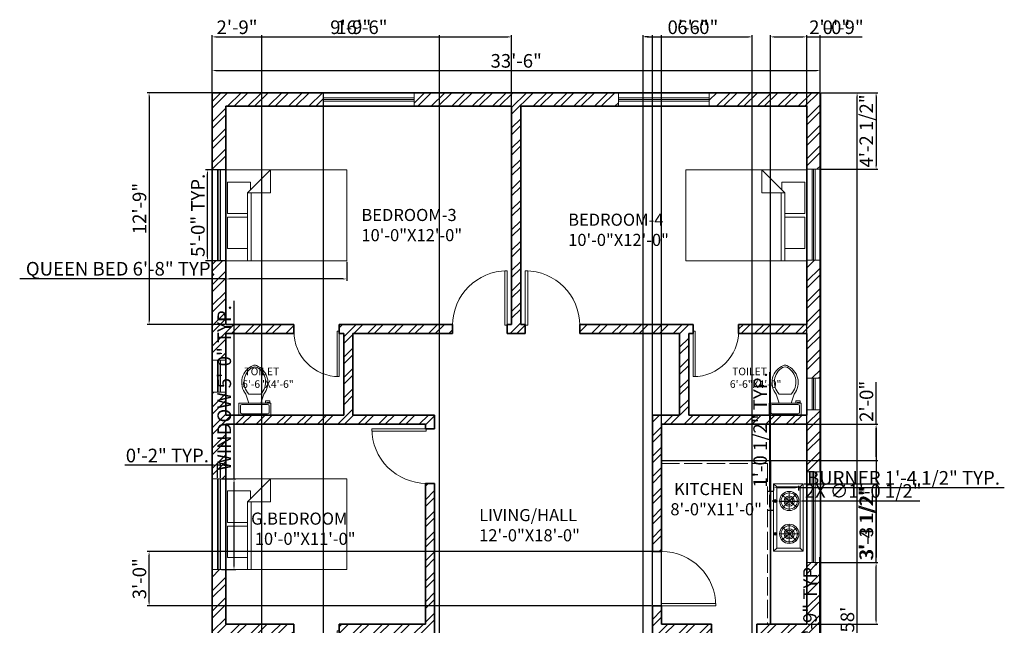
# Model space of a CAD drawing. Units: inches. Extents: x 73 to 724, y 1566 to 2355.
# Tile 2 of 2: x 73 to 724, y 1955 to 2355. Entities that reach past the tile are written whole.
import ezdxf

# ---------------------------------------------------------------- set-up
doc = ezdxf.new("R2010")
doc.units = ezdxf.units.IN
doc.linetypes.add('ACAD_ISO02W100', pattern=[15, 12, -3])
for name, color, linetype, lineweight in [('A-ANNO-DIMS', 2, 'Continuous', 18), ('A-AREA-IDEN', 7, 'Continuous', 18), ('A-DOOR', 4, 'Continuous', 18), ('A-EQPM', 8, 'Continuous', 18), ('A-FLOR-CASE', 9, 'Continuous', 25), ('A-FLOR-CASE-HIDN', 9, 'ACAD_ISO02W100', 13), ('A-FLOR-FIXT', 9, 'Continuous', 18), ('A-FURN', 9, 'Continuous', 18), ('A-GLAZ', 244, 'Continuous', 18), ('A-WALL', 7, 'Continuous', 35), ('A-WALL-PATT', 252, 'Continuous', 13)]:
    doc.layers.add(name, color=color, linetype=linetype, lineweight=lineweight)
doc.styles.get("Standard").update_dxf_attribs({"font": 'arial.ttf'})
doc.dimstyles.new('ISO-25', dxfattribs={"dimtxt": 9, "dimasz": 2.5, "dimexe": 1.25, "dimexo": 0.625, "dimtad": 1, "dimlunit": 3, "dimtxsty": 'Standard', "dimcen": 2.5, "dimadec": 0, "dimazin": 0, "dimtfac": 1, "dimtmove": 0, "dimatfit": 3, "dimfxl": 1, "dimarcsym": 0})

# ---------------------------------------------------------------- blocks, each defined once
blk = doc.blocks.new('*U3')
for p, q in [((0, 0), (0, -6)), ((-40, 0), (-40, -6))]:
    blk.add_line(p, q)
blk.add_lwpolyline([(0, 0), (0, 40), (-1.75, 40), (-1.75, 0)], close=True)
blk.add_arc((0, 0), 40, 90, 180)
blk = doc.blocks.new('*U4')
for p, q in [((0, 0), (0, -6)), ((40, 0), (40, -6))]:
    blk.add_line(p, q)
blk.add_lwpolyline([(0, 0), (0, 40), (1.75, 40), (1.75, 0)], close=True)
blk.add_arc((0, 0), 40, 0, 90)
blk = doc.blocks.new('*U5')
for p, q in [((0, 0), (0, 6)), ((40, 0), (40, 6))]:
    blk.add_line(p, q)
blk.add_lwpolyline([(0, 0), (0, -40), (1.75, -40), (1.75, 0)], close=True)
blk.add_arc((0, 0), 40, 270, 360)
blk = doc.blocks.new('*U6')
for p, q in [((0, 0), (0, 6)), ((40, 0), (40, 6))]:
    blk.add_line(p, q)
blk.add_lwpolyline([(0, 0), (0, -40), (1.75, -40), (1.75, 0)], close=True)
blk.add_arc((0, 0), 40, 270, 0)
blk = doc.blocks.new('*U8')
for p, q in [((-40, 0), (-40, 6)), ((0, 0), (0, 6))]:
    blk.add_line(p, q)
blk.add_lwpolyline([(0, 0), (0, -40), (-1.75, -40), (-1.75, 0)], close=True)
blk.add_arc((0, 0), 40, 180, 270)
blk = doc.blocks.new('*D9')
at = {"layer": 'A-ANNO-DIMS', "color": 0, "lineweight": -2, "transparency": 16777216}
for p, q in [((200.03, 2307.75), (200.03, 2323)), ((202.53, 2321.75), (599.53, 2321.75)), ((602.03, 2307.75), (602.03, 2323))]:
    blk.add_line(p, q, dxfattribs=at)
at = {"layer": 'A-ANNO-DIMS', "color": 0, "transparency": 16777216}
for points in [[(202.53, 2322.17), (202.53, 2321.34), (200.03, 2321.75)], [(599.53, 2322.17), (599.53, 2321.34), (602.03, 2321.75)]]:
    blk.add_solid(points, dxfattribs=at)
at = {"layer": 'Defpoints', "color": 0, "transparency": 16777216}
for p in [(602.03, 2321.75), (200.03, 2307.12), (602.03, 2307.12)]:
    blk.add_point(p, dxfattribs=at)
at = {"layer": 'A-ANNO-DIMS', "color": 0, "transparency": 16777216, "insert": (401.03, 2326.98), "char_height": 9, "attachment_point": 5}
blk.add_mtext('33\'-6"', dxfattribs=at)
blk = doc.blocks.new('*D10')
at = {"layer": 'A-ANNO-DIMS', "color": 0, "lineweight": -2, "transparency": 16777216}
for p, q in [((602.66, 2307.12), (627.57, 2307.12)), ((626.32, 1613.62), (626.32, 2304.62)), ((602.66, 1611.12), (627.57, 1611.12))]:
    blk.add_line(p, q, dxfattribs=at)
at = {"layer": 'A-ANNO-DIMS', "color": 0, "transparency": 16777216}
for points in [[(625.9, 2304.62), (626.74, 2304.62), (626.32, 2307.12)], [(625.9, 1613.62), (626.74, 1613.62), (626.32, 1611.12)]]:
    blk.add_solid(points, dxfattribs=at)
at = {"layer": 'Defpoints', "color": 0, "transparency": 16777216}
for p in [(602.03, 2307.12), (626.32, 2307.12), (602.03, 1611.12)]:
    blk.add_point(p, dxfattribs=at)
at = {"layer": 'A-ANNO-DIMS', "color": 0, "transparency": 16777216, "insert": (621.1, 1959.12), "char_height": 9, "attachment_point": 5, "rotation": 90}
blk.add_mtext("58'", dxfattribs=at)
blk = doc.blocks.new('Bed - Queen')
for p, q in [((0, -80.00003), (0, 0)), ((0, 0), (59.99999, 0)), ((59.99999, 0), (59.99999, -80.00003)), ((7.99999, -1.2), (28.79998, -1.2)), ((7.99999, -14.4), (7.99999, -1.2)), ((28.79998, -1.2), (28.79998, -14.4)), ((31.19999, -1.2), (51.99999, -1.2)), ((31.19999, -14.4), (31.19999, -1.2)), ((51.99999, -1.2), (51.99999, -16.4)), ((0, -14.4), (44.8, -14.4)), ((44.8, -16.8), (0, -16.8)), ((59.99999, -29.6), (44.8, -14.4)), ((44.8, -14.4), (44.8, -29.6)), ((51.99999, -16.4), (46.79936, -16.4)), ((44.8, -29.6), (59.99999, -29.6)), ((59.99999, -80.00003), (0, -80.00003))]:
    blk.add_line(p, q)
blk = doc.blocks.new('*U13')
for p, q in [((9.5, -6), (9.5, -2)), ((-10, -8.5), (-8, -8.5)), ((-10, -9.5), (-10, -8.5)), ((-7, -9.5), (-10, -9.5)), ((-8, -8.5), (-8, -8)), ((-7, -8), (-7, -9.5)), ((-4, -8), (-6, -14)), ((4, -8), (6, -14)), ((4, -14), (-4, -14))]:
    blk.add_line(p, q)
blk.add_lwpolyline([(10.5, -8), (10.5, 0), (-10.5, 0), (-10.5, -8)], close=True)
for points in [[(-9.5, -2), (-9.5, -6)], [(8.5, -1), (-8.5, -1)], [(-8.5, -7), (8.5, -7)]]:
    blk.add_lwpolyline(points)
for centre, radius, start, end in [((-8.62, -1.88), 0.884, 81.8699, 188.1301), ((-8.62, -6.12), 0.884, 171.8699, 278.1301), ((8.62, -1.88), 0.884, 351.8699, 98.1301), ((8.62, -6.12), 0.884, 261.8699, 8.1301), ((3.52, -21.58), 12.17, 141.46911, 247.97143), ((4.2, -21.82), 11.33, 136.36773, 238.94682), ((-3.52, -21.58), 12.17, 292.02843, 38.53071), ((-4.2, -21.82), 11.33, 301.05301, 43.63209), ((0, -27.88), 4, 245.73182, 294.26817), ((0, -29), 4, 254.86053, 285.13947)]:
    blk.add_arc(centre, radius, start, end)
blk = doc.blocks.new('WIN-GLAZING-60IN')
for p, q in [((0, 2), (60, 2)), ((0, 1), (60, 1)), ((0, 0), (60, 0))]:
    blk.add_line(p, q)
blk = doc.blocks.new('WIN-GLAZING-21IN')
for p, q in [((0, 21), (0, 0)), ((1, 21), (1, 0)), ((2, 21), (2, 0))]:
    blk.add_line(p, q)
blk = doc.blocks.new('COOKTOP-BURNER-AND-CONTROL')
for p, q in [((0.78, 7.28), (0.78, 5.37)), ((1.18, 7.28), (1.18, 5.37)), ((15.23, 2.35), (5.36, 10.38)), ((5.73, 1.93), (14.86, 10.8)), ((10.3, 12.73), (10.3, 0)), ((3.93, 6.36), (16.66, 6.36))]:
    blk.add_line(p, q)
for centre, radius in [((0.98, 6.33), 0.976), ((10.3, 6.36), 6.36), ((10.3, 6.36), 5.36), ((10.3, 6.36), 3.36), ((10.3, 6.36), 2.36)]:
    blk.add_circle(centre, radius)
for start, end in [(122.10123, 237.89877), (302.10123, 57.89877)]:
    blk.add_arc((0.98, 6.33), 0.376, start, end)
blk = doc.blocks.new('*D19')
at = {"layer": 'A-ANNO-DIMS', "color": 0, "lineweight": -2, "transparency": 16777216}
for p, q in [((214.53, 2052.12), (214.53, 2169.76)), ((206.16, 2052.12), (215.78, 2052.12)), ((214.53, 1994.62), (214.53, 2049.62)), ((206.16, 1992.12), (215.78, 1992.12))]:
    blk.add_line(p, q, dxfattribs=at)
at = {"layer": 'A-ANNO-DIMS', "color": 0, "transparency": 16777216}
for points in [[(214.12, 2049.62), (214.95, 2049.62), (214.53, 2052.12)], [(214.12, 1994.62), (214.95, 1994.62), (214.53, 1992.12)]]:
    blk.add_solid(points, dxfattribs=at)
at = {"layer": 'Defpoints', "color": 0, "transparency": 16777216}
for p in [(205.53, 2052.12), (214.53, 2052.12), (205.53, 1992.12)]:
    blk.add_point(p, dxfattribs=at)
at = {"layer": 'A-ANNO-DIMS', "color": 0, "transparency": 16777216, "insert": (209.25, 2112.19), "char_height": 9, "attachment_point": 5, "rotation": 90}
blk.add_mtext('WINDOW 5\'-0" TYP.', dxfattribs=at)
blk = doc.blocks.new('*D20')
at = {"layer": 'A-ANNO-DIMS', "color": 0, "lineweight": -2, "transparency": 16777216}
for p, q in [((201.03, 2061.12), (142.43, 2061.12)), ((203.53, 2052.75), (203.53, 2062.37)), ((205.53, 2061.12), (203.53, 2061.12)), ((205.53, 2052.75), (205.53, 2062.37)), ((208.03, 2061.12), (210.53, 2061.12))]:
    blk.add_line(p, q, dxfattribs=at)
at = {"layer": 'A-ANNO-DIMS', "color": 0, "transparency": 16777216}
for points in [[(201.03, 2061.54), (201.03, 2060.71), (203.53, 2061.12)], [(208.03, 2061.54), (208.03, 2060.71), (205.53, 2061.12)]]:
    blk.add_solid(points, dxfattribs=at)
at = {"layer": 'Defpoints', "color": 0, "transparency": 16777216}
for p in [(203.53, 2061.12), (203.53, 2052.12), (205.53, 2052.12)]:
    blk.add_point(p, dxfattribs=at)
at = {"layer": 'A-ANNO-DIMS', "color": 0, "transparency": 16777216, "insert": (170.48, 2066.34), "char_height": 9, "attachment_point": 5}
blk.add_mtext('0\'-2" TYP.', dxfattribs=at)
blk = doc.blocks.new('*D21')
at = {"layer": 'A-ANNO-DIMS', "color": 0, "lineweight": -2, "transparency": 16777216}
for p, q in [((601.68, 1882.62), (601.68, 2000.26)), ((599.16, 1882.62), (602.93, 1882.62)), ((601.68, 1864.12), (601.68, 1880.12)), ((599.16, 1861.62), (602.93, 1861.62))]:
    blk.add_line(p, q, dxfattribs=at)
at = {"layer": 'A-ANNO-DIMS', "color": 0, "transparency": 16777216}
for points in [[(601.27, 1880.12), (602.1, 1880.12), (601.68, 1882.62)], [(601.27, 1864.12), (602.1, 1864.12), (601.68, 1861.62)]]:
    blk.add_solid(points, dxfattribs=at)
at = {"layer": 'Defpoints', "color": 0, "transparency": 16777216}
for p in [(598.53, 1882.62), (601.68, 1882.62), (598.53, 1861.62)]:
    blk.add_point(p, dxfattribs=at)
at = {"layer": 'A-ANNO-DIMS', "color": 0, "transparency": 16777216, "insert": (596.4, 1942.69), "char_height": 9, "attachment_point": 5, "rotation": 90}
blk.add_mtext('WINDOW 1\'-9" TYP.', dxfattribs=at)
blk = doc.blocks.new('*D23')
at = {"layer": 'A-ANNO-DIMS', "color": 0, "lineweight": -2, "transparency": 16777216}
for p, q in [((209.03, 2195.5), (209.03, 2182.87)), ((289.03, 2195.5), (289.03, 2182.87)), ((209.03, 2184.12), (72.89, 2184.12)), ((286.53, 2184.12), (211.53, 2184.12))]:
    blk.add_line(p, q, dxfattribs=at)
at = {"layer": 'A-ANNO-DIMS', "color": 0, "transparency": 16777216}
for points in [[(211.53, 2184.54), (211.53, 2183.71), (209.03, 2184.12)], [(286.53, 2184.54), (286.53, 2183.71), (289.03, 2184.12)]]:
    blk.add_solid(points, dxfattribs=at)
at = {"layer": 'Defpoints', "color": 0, "transparency": 16777216}
for p in [(209.03, 2196.12), (289.03, 2196.12), (209.03, 2184.12)]:
    blk.add_point(p, dxfattribs=at)
at = {"layer": 'A-ANNO-DIMS', "color": 0, "transparency": 16777216, "insert": (139.71, 2189.68), "char_height": 9, "attachment_point": 5}
blk.add_mtext('QUEEN BED 6\'-8" TYP.', dxfattribs=at)
blk = doc.blocks.new('*D24')
at = {"layer": 'A-ANNO-DIMS', "color": 0, "lineweight": -2, "transparency": 16777216}
for p, q in [((208.41, 2256.12), (195.78, 2256.12)), ((197.03, 2198.62), (197.03, 2253.62)), ((208.41, 2196.12), (195.78, 2196.12))]:
    blk.add_line(p, q, dxfattribs=at)
at = {"layer": 'A-ANNO-DIMS', "color": 0, "transparency": 16777216}
for points in [[(196.62, 2253.62), (197.45, 2253.62), (197.03, 2256.12)], [(196.62, 2198.62), (197.45, 2198.62), (197.03, 2196.12)]]:
    blk.add_solid(points, dxfattribs=at)
at = {"layer": 'Defpoints', "color": 0, "transparency": 16777216}
for p in [(197.03, 2256.12), (209.03, 2256.12), (209.03, 2196.12)]:
    blk.add_point(p, dxfattribs=at)
at = {"layer": 'A-ANNO-DIMS', "color": 0, "transparency": 16777216, "insert": (191.81, 2226.12), "char_height": 9, "attachment_point": 5, "rotation": 90}
blk.add_mtext('5\'-0" TYP.', dxfattribs=at)
blk = doc.blocks.new('*D25')
at = {"layer": 'A-ANNO-DIMS', "color": 0, "lineweight": -2, "transparency": 16777216}
for p, q in [((571.19, 2044.43), (571.19, 2047.56)), ((573.69, 2046.31), (585.35, 2046.31)), ((587.85, 2044.43), (587.85, 2047.56)), ((587.85, 2046.31), (723.62, 2046.31))]:
    blk.add_line(p, q, dxfattribs=at)
at = {"layer": 'A-ANNO-DIMS', "color": 0, "transparency": 16777216}
for points in [[(573.69, 2046.72), (573.69, 2045.89), (571.19, 2046.31)], [(585.35, 2046.72), (585.35, 2045.89), (587.85, 2046.31)]]:
    blk.add_solid(points, dxfattribs=at)
at = {"layer": 'Defpoints', "color": 0, "transparency": 16777216}
for p in [(571.19, 2043.81), (587.85, 2046.31), (587.85, 2043.81)]:
    blk.add_point(p, dxfattribs=at)
at = {"layer": 'A-ANNO-DIMS', "color": 0, "transparency": 16777216, "insert": (656.98, 2051.58), "char_height": 9, "attachment_point": 5}
blk.add_mtext('BURNER 1\'-4 1/2" TYP.', dxfattribs=at)
blk = doc.blocks.new('*D26')
at = {"layer": 'A-ANNO-DIMS', "color": 0, "lineweight": -2, "transparency": 16777216}
for p, q in [((568.69, 2043.81), (568.69, 2122.54)), ((570.56, 2043.81), (567.44, 2043.81)), ((568.69, 2033.58), (568.69, 2041.31)), ((570.56, 2031.08), (567.44, 2031.08))]:
    blk.add_line(p, q, dxfattribs=at)
at = {"layer": 'A-ANNO-DIMS', "color": 0, "transparency": 16777216}
for points in [[(568.27, 2041.31), (569.1, 2041.31), (568.69, 2043.81)], [(568.27, 2033.58), (569.1, 2033.58), (568.69, 2031.08)]]:
    blk.add_solid(points, dxfattribs=at)
at = {"layer": 'Defpoints', "color": 0, "transparency": 16777216}
for p in [(568.69, 2043.81), (571.19, 2043.81), (571.19, 2031.08)]:
    blk.add_point(p, dxfattribs=at)
at = {"layer": 'A-ANNO-DIMS', "color": 0, "transparency": 16777216, "insert": (563.41, 2084.42), "char_height": 9, "attachment_point": 5, "rotation": 90}
blk.add_mtext('1\'-0 1/2" TYP.', dxfattribs=at)
blk = doc.blocks.new('*D29')
at = {"layer": 'A-ANNO-DIMS', "color": 0, "lineweight": -2, "transparency": 16777216}
for p, q in [((200.03, 2307.75), (200.03, 2345.22)), ((202.53, 2343.97), (395.53, 2343.97)), ((398.03, 2298.75), (398.03, 2345.22))]:
    blk.add_line(p, q, dxfattribs=at)
at = {"layer": 'A-ANNO-DIMS', "color": 0, "transparency": 16777216}
for points in [[(202.53, 2344.39), (202.53, 2343.56), (200.03, 2343.97)], [(395.53, 2344.39), (395.53, 2343.56), (398.03, 2343.97)]]:
    blk.add_solid(points, dxfattribs=at)
at = {"layer": 'Defpoints', "color": 0, "transparency": 16777216}
for p in [(398.03, 2343.97), (200.03, 2307.12), (398.03, 2298.12)]:
    blk.add_point(p, dxfattribs=at)
at = {"layer": 'A-ANNO-DIMS', "color": 0, "transparency": 16777216, "insert": (299.03, 2349.19), "char_height": 9, "attachment_point": 5}
blk.add_mtext('16\'-6"', dxfattribs=at)
blk = doc.blocks.new('*D30')
at = {"layer": 'A-ANNO-DIMS', "color": 0, "lineweight": -2, "transparency": 16777216}
for p, q in [((199.41, 2307.12), (157.17, 2307.12)), ((158.42, 2304.62), (158.42, 2156.62)), ((208.41, 2154.12), (157.17, 2154.12))]:
    blk.add_line(p, q, dxfattribs=at)
at = {"layer": 'A-ANNO-DIMS', "color": 0, "transparency": 16777216}
for points in [[(158, 2304.62), (158.84, 2304.62), (158.42, 2307.12)], [(158, 2156.62), (158.84, 2156.62), (158.42, 2154.12)]]:
    blk.add_solid(points, dxfattribs=at)
at = {"layer": 'Defpoints', "color": 0, "transparency": 16777216}
for p in [(200.03, 2307.12), (158.42, 2154.12), (209.03, 2154.12)]:
    blk.add_point(p, dxfattribs=at)
at = {"layer": 'A-ANNO-DIMS', "color": 0, "transparency": 16777216, "insert": (153.2, 2230.62), "char_height": 9, "attachment_point": 5, "rotation": 90}
blk.add_mtext('12\'-9"', dxfattribs=at)
blk = doc.blocks.new('*D32')
at = {"layer": 'A-ANNO-DIMS', "color": 0, "lineweight": -2, "transparency": 16777216}
for p, q in [((569.03, 1956.75), (569.03, 2345.22)), ((571.53, 2343.97), (590.53, 2343.97)), ((593.03, 1956.75), (593.03, 2345.22)), ((593.03, 2343.97), (620.86, 2343.97))]:
    blk.add_line(p, q, dxfattribs=at)
at = {"layer": 'A-ANNO-DIMS', "color": 0, "transparency": 16777216}
for points in [[(571.53, 2344.39), (571.53, 2343.56), (569.03, 2343.97)], [(590.53, 2344.39), (590.53, 2343.56), (593.03, 2343.97)]]:
    blk.add_solid(points, dxfattribs=at)
at = {"layer": 'Defpoints', "color": 0, "transparency": 16777216}
for p in [(593.03, 2343.97), (569.03, 1956.12), (593.03, 1956.12)]:
    blk.add_point(p, dxfattribs=at)
at = {"layer": 'A-ANNO-DIMS', "color": 0, "transparency": 16777216, "insert": (608.2, 2349.19), "char_height": 9, "attachment_point": 5}
blk.add_mtext('2\'-0"', dxfattribs=at)
blk = doc.blocks.new('*D33')
at = {"layer": 'A-ANNO-DIMS', "color": 0, "lineweight": -2, "transparency": 16777216}
for p, q in [((490.41, 2004.12), (157.17, 2004.12)), ((158.42, 1970.62), (158.42, 2001.62)), ((490.41, 1968.12), (157.17, 1968.12))]:
    blk.add_line(p, q, dxfattribs=at)
at = {"layer": 'A-ANNO-DIMS', "color": 0, "transparency": 16777216}
for points in [[(158, 2001.62), (158.84, 2001.62), (158.42, 2004.12)], [(158, 1970.62), (158.84, 1970.62), (158.42, 1968.12)]]:
    blk.add_solid(points, dxfattribs=at)
at = {"layer": 'Defpoints', "color": 0, "transparency": 16777216}
for p in [(158.42, 2004.12), (491.03, 2004.12), (491.03, 1968.12)]:
    blk.add_point(p, dxfattribs=at)
at = {"layer": 'A-ANNO-DIMS', "color": 0, "transparency": 16777216, "insert": (153.2, 1986.12), "char_height": 9, "attachment_point": 5, "rotation": 90}
blk.add_mtext('3\'-0"', dxfattribs=at)
blk = doc.blocks.new('*D34')
at = {"layer": 'A-ANNO-DIMS', "color": 0, "lineweight": -2, "transparency": 16777216}
for p, q in [((638.88, 2088.12), (638.88, 2115.95)), ((497.66, 2088.12), (640.13, 2088.12)), ((638.88, 2066.62), (638.88, 2085.62)), ((497.66, 2064.12), (640.13, 2064.12))]:
    blk.add_line(p, q, dxfattribs=at)
at = {"layer": 'A-ANNO-DIMS', "color": 0, "transparency": 16777216}
for points in [[(638.47, 2085.62), (639.3, 2085.62), (638.88, 2088.12)], [(638.47, 2066.62), (639.3, 2066.62), (638.88, 2064.12)]]:
    blk.add_solid(points, dxfattribs=at)
at = {"layer": 'Defpoints', "color": 0, "transparency": 16777216}
for p in [(497.03, 2088.12), (638.88, 2088.12), (497.03, 2064.12)]:
    blk.add_point(p, dxfattribs=at)
at = {"layer": 'A-ANNO-DIMS', "color": 0, "transparency": 16777216, "insert": (633.66, 2103.29), "char_height": 9, "attachment_point": 5, "rotation": 90}
blk.add_mtext('2\'-0"', dxfattribs=at)
blk = doc.blocks.new('*D36')
at = {"layer": 'A-ANNO-DIMS', "color": 0, "lineweight": -2, "transparency": 16777216}
for p, q in [((233.03, 1719.75), (233.03, 2345.22)), ((235.53, 2343.97), (347.77, 2343.97)), ((350.27, 1719.75), (350.27, 2345.22))]:
    blk.add_line(p, q, dxfattribs=at)
at = {"layer": 'A-ANNO-DIMS', "color": 0, "transparency": 16777216}
for points in [[(235.53, 2344.39), (235.53, 2343.56), (233.03, 2343.97)], [(347.77, 2344.39), (347.77, 2343.56), (350.27, 2343.97)]]:
    blk.add_solid(points, dxfattribs=at)
at = {"layer": 'Defpoints', "color": 0, "transparency": 16777216}
for p in [(350.27, 2343.97), (233.03, 1719.12), (350.27, 1719.12)]:
    blk.add_point(p, dxfattribs=at)
at = {"layer": 'A-ANNO-DIMS', "color": 0, "transparency": 16777216, "insert": (291.65, 2349.19), "char_height": 9, "attachment_point": 5}
blk.add_mtext('9\'-9"', dxfattribs=at)
blk = doc.blocks.new('*D37')
at = {"layer": 'A-ANNO-DIMS', "color": 0, "lineweight": -2, "transparency": 16777216}
for p, q in [((200.03, 1710.75), (200.03, 2345.22)), ((202.53, 2343.97), (230.53, 2343.97)), ((233.03, 1719.75), (233.03, 2345.22))]:
    blk.add_line(p, q, dxfattribs=at)
at = {"layer": 'A-ANNO-DIMS', "color": 0, "transparency": 16777216}
for points in [[(202.53, 2344.39), (202.53, 2343.56), (200.03, 2343.97)], [(230.53, 2344.39), (230.53, 2343.56), (233.03, 2343.97)]]:
    blk.add_solid(points, dxfattribs=at)
at = {"layer": 'Defpoints', "color": 0, "transparency": 16777216}
for p in [(233.03, 2343.97), (233.03, 1719.12), (200.03, 1710.12)]:
    blk.add_point(p, dxfattribs=at)
at = {"layer": 'A-ANNO-DIMS', "color": 0, "transparency": 16777216, "insert": (216.53, 2349.19), "char_height": 9, "attachment_point": 5}
blk.add_mtext('2\'-9"', dxfattribs=at)
blk = doc.blocks.new('*D38')
at = {"layer": 'A-ANNO-DIMS', "color": 0, "lineweight": -2, "transparency": 16777216}
for p, q in [((200.03, 2306.5), (200.03, 1573.02)), ((273.53, 2306.5), (273.53, 1573.02)), ((202.53, 1574.27), (271.03, 1574.27))]:
    blk.add_line(p, q, dxfattribs=at)
at = {"layer": 'A-ANNO-DIMS', "color": 0, "transparency": 16777216}
for points in [[(202.53, 1574.69), (202.53, 1573.86), (200.03, 1574.27)], [(271.03, 1574.69), (271.03, 1573.86), (273.53, 1574.27)]]:
    blk.add_solid(points, dxfattribs=at)
at = {"layer": 'Defpoints', "color": 0, "transparency": 16777216}
for p in [(200.03, 2307.12), (273.53, 2307.12), (273.53, 1574.27)]:
    blk.add_point(p, dxfattribs=at)
at = {"layer": 'A-ANNO-DIMS', "color": 0, "transparency": 16777216, "insert": (236.78, 1579.55), "char_height": 9, "attachment_point": 5}
blk.add_mtext('6\'-1 1/2"', dxfattribs=at)
blk = doc.blocks.new('*D39')
at = {"layer": 'A-ANNO-DIMS', "color": 0, "lineweight": -2, "transparency": 16777216}
for p, q in [((602.66, 2307.12), (640.13, 2307.12)), ((638.88, 2304.62), (638.88, 2259.09)), ((602.66, 2256.59), (640.13, 2256.59))]:
    blk.add_line(p, q, dxfattribs=at)
at = {"layer": 'A-ANNO-DIMS', "color": 0, "transparency": 16777216}
for points in [[(638.47, 2304.62), (639.3, 2304.62), (638.88, 2307.12)], [(638.47, 2259.09), (639.3, 2259.09), (638.88, 2256.59)]]:
    blk.add_solid(points, dxfattribs=at)
at = {"layer": 'Defpoints', "color": 0, "transparency": 16777216}
for p in [(602.03, 2307.12), (602.03, 2256.59), (638.88, 2256.59)]:
    blk.add_point(p, dxfattribs=at)
at = {"layer": 'A-ANNO-DIMS', "color": 0, "transparency": 16777216, "insert": (633.61, 2281.85), "char_height": 9, "attachment_point": 5, "rotation": 90}
blk.add_mtext('4\'-2 1/2"', dxfattribs=at)
blk = doc.blocks.new('*D41')
at = {"layer": 'A-ANNO-DIMS', "color": 0, "lineweight": -2, "transparency": 16777216}
for p, q in [((593.66, 2088.12), (640.13, 2088.12)), ((638.88, 2085.62), (638.88, 2051.29)), ((591.39, 2048.79), (640.13, 2048.79)), ((638.88, 2048.79), (638.88, 2000.15))]:
    blk.add_line(p, q, dxfattribs=at)
at = {"layer": 'A-ANNO-DIMS', "color": 0, "transparency": 16777216}
for points in [[(638.47, 2085.62), (639.3, 2085.62), (638.88, 2088.12)], [(638.47, 2051.29), (639.3, 2051.29), (638.88, 2048.79)]]:
    blk.add_solid(points, dxfattribs=at)
at = {"layer": 'Defpoints', "color": 0, "transparency": 16777216}
for p in [(593.03, 2088.12), (590.76, 2048.79), (638.88, 2048.79)]:
    blk.add_point(p, dxfattribs=at)
at = {"layer": 'A-ANNO-DIMS', "color": 0, "transparency": 16777216, "insert": (633.6, 2023.22), "char_height": 9, "attachment_point": 5, "rotation": 90}
blk.add_mtext('3\'-3 1/2"', dxfattribs=at)
blk = doc.blocks.new('*D42')
at = {"layer": 'A-ANNO-DIMS', "color": 0, "lineweight": -2, "transparency": 16777216}
for p, q in [((593.03, 2057.41), (593.03, 2345.22)), ((595.53, 2343.97), (599.53, 2343.97)), ((602.03, 2057.41), (602.03, 2345.22)), ((602.03, 2343.97), (629.71, 2343.97))]:
    blk.add_line(p, q, dxfattribs=at)
at = {"layer": 'A-ANNO-DIMS', "color": 0, "transparency": 16777216}
for points in [[(595.53, 2344.39), (595.53, 2343.56), (593.03, 2343.97)], [(599.53, 2344.39), (599.53, 2343.56), (602.03, 2343.97)]]:
    blk.add_solid(points, dxfattribs=at)
at = {"layer": 'Defpoints', "color": 0, "transparency": 16777216}
for p in [(602.03, 2343.97), (593.03, 2056.78), (602.03, 2056.78)]:
    blk.add_point(p, dxfattribs=at)
at = {"layer": 'A-ANNO-DIMS', "color": 0, "transparency": 16777216, "insert": (617.12, 2349.19), "char_height": 9, "attachment_point": 5}
blk.add_mtext('0\'-9"', dxfattribs=at)
blk = doc.blocks.new('*D43')
at = {"layer": 'A-ANNO-DIMS', "color": 0, "lineweight": -2, "transparency": 16777216}
for p, q in [((488.53, 2343.97), (486.03, 2343.97)), ((491.03, 1968.75), (491.03, 2345.22)), ((491.03, 2343.97), (497.03, 2343.97)), ((497.03, 1968.75), (497.03, 2345.22)), ((499.53, 2343.97), (527.21, 2343.97))]:
    blk.add_line(p, q, dxfattribs=at)
at = {"layer": 'A-ANNO-DIMS', "color": 0, "transparency": 16777216}
for points in [[(488.53, 2344.39), (488.53, 2343.56), (491.03, 2343.97)], [(499.53, 2344.39), (499.53, 2343.56), (497.03, 2343.97)]]:
    blk.add_solid(points, dxfattribs=at)
at = {"layer": 'Defpoints', "color": 0, "transparency": 16777216}
for p in [(497.03, 2343.97), (491.03, 1968.12), (497.03, 1968.12)]:
    blk.add_point(p, dxfattribs=at)
at = {"layer": 'A-ANNO-DIMS', "color": 0, "transparency": 16777216, "insert": (514.62, 2349.19), "char_height": 9, "attachment_point": 5}
blk.add_mtext('0\'-6"', dxfattribs=at)
blk = doc.blocks.new('*D44')
at = {"layer": 'A-ANNO-DIMS', "color": 0, "lineweight": -2, "transparency": 16777216}
for p, q in [((638.88, 1996.78), (638.88, 2045.42)), ((602.66, 1996.78), (640.13, 1996.78)), ((638.88, 1958.62), (638.88, 1994.28)), ((593.66, 1956.12), (640.13, 1956.12))]:
    blk.add_line(p, q, dxfattribs=at)
at = {"layer": 'A-ANNO-DIMS', "color": 0, "transparency": 16777216}
for points in [[(638.47, 1994.28), (639.3, 1994.28), (638.88, 1996.78)], [(638.47, 1958.62), (639.3, 1958.62), (638.88, 1956.12)]]:
    blk.add_solid(points, dxfattribs=at)
at = {"layer": 'Defpoints', "color": 0, "transparency": 16777216}
for p in [(602.03, 1996.78), (638.88, 1996.78), (593.03, 1956.12)]:
    blk.add_point(p, dxfattribs=at)
at = {"layer": 'A-ANNO-DIMS', "color": 0, "transparency": 16777216, "insert": (633.6, 2022.35), "char_height": 9, "attachment_point": 5, "rotation": 90}
blk.add_mtext('3\'-4 1/2"', dxfattribs=at)
blk = doc.blocks.new('*D46')
at = {"layer": 'A-ANNO-DIMS', "color": 0, "lineweight": -2, "transparency": 16777216}
for p, q in [((485.03, 1686.75), (485.03, 2345.22)), ((487.53, 2343.97), (554.53, 2343.97)), ((557.03, 1686.75), (557.03, 2345.22))]:
    blk.add_line(p, q, dxfattribs=at)
at = {"layer": 'A-ANNO-DIMS', "color": 0, "transparency": 16777216}
for points in [[(487.53, 2344.39), (487.53, 2343.56), (485.03, 2343.97)], [(554.53, 2344.39), (554.53, 2343.56), (557.03, 2343.97)]]:
    blk.add_solid(points, dxfattribs=at)
at = {"layer": 'Defpoints', "color": 0, "transparency": 16777216}
for p in [(557.03, 2343.97), (485.03, 1686.12), (557.03, 1686.12)]:
    blk.add_point(p, dxfattribs=at)
at = {"layer": 'A-ANNO-DIMS', "color": 0, "transparency": 16777216, "insert": (521.03, 2349.19), "char_height": 9, "attachment_point": 5}
blk.add_mtext('6\'-0"', dxfattribs=at)
blk = doc.blocks.new('*D47')
at = {"layer": 'A-ANNO-DIMS', "color": 0, "lineweight": -2, "transparency": 16777216}
for p, q in [((572.62, 2037.44), (570.12, 2037.44)), ((575.12, 2037.44), (587.85, 2037.44)), ((667.8, 2037.45), (590.35, 2037.44))]:
    blk.add_line(p, q, dxfattribs=at)
at = {"layer": 'A-ANNO-DIMS', "color": 0, "transparency": 16777216}
for points in [[(572.62, 2037.86), (572.62, 2037.02), (575.12, 2037.44)], [(590.35, 2037.86), (590.35, 2037.03), (587.85, 2037.44)]]:
    blk.add_solid(points, dxfattribs=at)
at = {"layer": 'Defpoints', "color": 0, "transparency": 16777216}
for p in [(575.12, 2037.44), (587.85, 2037.44)]:
    blk.add_point(p, dxfattribs=at)
at = {"layer": 'A-ANNO-DIMS', "color": 0, "transparency": 16777216, "insert": (630.33, 2042.92), "char_height": 9, "attachment_point": 5, "rotation": 0.00374}
blk.add_mtext('2X ∅1\'-0 1/2"', dxfattribs=at)

msp = doc.modelspace()

# ---------------------------------------------------------------- hatches: boundary and pattern name
at = {"layer": 'A-WALL-PATT'}
h = msp.add_hatch(dxfattribs=at)
h.set_pattern_fill('ANSI32', color=256)
h.paths.add_polyline_path([(209.035, 2088.122), (341.035, 2088.122), (341.035, 2085.122), (341.635, 2085.122), (347.035, 2085.122), (347.035, 2094.122), (293.035, 2094.122), (293.035, 2148.122), (359.035, 2148.122), (359.035, 2154.122), (284.035, 2154.122), (284.035, 2149.622), (284.035, 2148.122), (287.035, 2148.122), (287.035, 2094.122), (209.035, 2094.122), (209.035, 2109.443), (200.035, 2109.443), (200.035, 2052.122), (209.035, 2052.122)])
h.paths.add_polyline_path([(347.035, 2049.122), (341.035, 2049.122), (341.035, 1956.122), (284.035, 1956.122), (284.035, 1951.622), (284.035, 1950.122), (287.035, 1950.122), (287.035, 1896.122), (209.035, 1896.122), (209.035, 1910.964), (200.035, 1910.964), (200.035, 1863.122), (209.035, 1863.122), (209.035, 1887.122), (295.787, 1887.122), (295.787, 1896.122), (293.035, 1896.122), (293.035, 1950.122), (347.035, 1950.122)])
h.paths.add_polyline_path([(209.035, 1992.122), (200.035, 1992.122), (200.035, 1931.964), (209.035, 1931.964), (209.035, 1950.122), (254.035, 1950.122), (254.035, 1956.122), (209.035, 1956.122)], flags=17)
h.paths.add_polyline_path([(344.268, 1896.122), (335.891, 1896.122), (335.891, 1887.122), (338.268, 1887.122), (338.268, 1836.258), (347.268, 1836.258), (347.268, 1842.258), (344.268, 1842.258)])
h.paths.add_polyline_path([(449.035, 1842.122), (452.035, 1842.122), (452.035, 1848.122), (443.035, 1848.122), (443.035, 1808.396), (441.494, 1808.396), (441.494, 1802.396), (443.035, 1802.396), (443.035, 1719.122), (350.268, 1719.122), (350.268, 1710.122), (443.035, 1710.122), (443.035, 1611.122), (449.035, 1611.122), (449.035, 1677.122), (485.035, 1677.122), (485.035, 1686.122), (449.035, 1686.122)])
h.paths.add_polyline_path([(407.035, 1848.122), (401.035, 1848.122), (401.035, 1842.258), (395.268, 1842.258), (395.268, 1836.258), (401.035, 1836.258), (401.035, 1802.396), (409.436, 1802.396), (409.436, 1808.396), (407.035, 1808.396)], flags=17)
h.paths.add_polyline_path([(497.035, 1896.122), (593.035, 1896.122), (593.035, 1882.622), (602.035, 1882.622), (602.035, 1908.472), (593.035, 1908.472), (593.035, 1902.122), (527.035, 1902.122), (527.035, 1950.122), (530.035, 1950.122), (530.035, 1956.122), (497.035, 1956.122), (497.035, 1968.122), (491.035, 1968.122), (491.035, 1950.122), (521.035, 1950.122), (521.035, 1902.122), (491.035, 1902.122), (491.035, 1848.122), (488.035, 1848.122), (488.035, 1842.122), (500.035, 1842.122), (500.035, 1848.122), (497.035, 1848.122)])
h.paths.add_polyline_path([(602.035, 1861.622), (593.035, 1861.622), (593.035, 1848.122), (530.035, 1848.122), (530.035, 1842.122), (593.035, 1842.122), (593.035, 1799.304), (602.035, 1799.304)])
h.paths.add_polyline_path([(602.035, 1739.304), (593.035, 1739.304), (593.035, 1686.122), (557.035, 1686.122), (557.035, 1677.122), (593.035, 1677.122), (593.035, 1611.122), (602.035, 1611.122)])
h.paths.add_polyline_path([(209.035, 1743.122), (200.035, 1743.122), (200.035, 1710.122), (233.035, 1710.122), (233.035, 1719.122), (209.035, 1719.122)])
h.paths.add_polyline_path([(602.035, 1996.783), (593.035, 1996.783), (593.035, 1956.122), (560.035, 1956.122), (560.035, 1950.122), (593.035, 1950.122), (593.035, 1929.472), (602.035, 1929.472)])
h.paths.add_polyline_path([(602.035, 2097.565), (593.035, 2097.565), (593.035, 2094.122), (515.035, 2094.122), (515.035, 2148.122), (518.035, 2148.122), (518.035, 2154.122), (443.035, 2154.122), (443.035, 2148.122), (509.035, 2148.122), (509.035, 2094.122), (491.035, 2094.122), (491.035, 2004.122), (497.035, 2004.122), (497.035, 2088.122), (593.035, 2088.122), (593.035, 2056.783), (602.035, 2056.783)])
h.paths.add_polyline_path([(602.035, 2196.587), (593.035, 2196.587), (593.035, 2154.122), (548.035, 2154.122), (548.035, 2148.122), (593.035, 2148.122), (593.035, 2118.565), (602.035, 2118.565)])
h.paths.add_polyline_path([(602.035, 2307.122), (528.535, 2307.122), (528.535, 2298.122), (593.035, 2298.122), (593.035, 2256.587), (602.035, 2256.587)])
h.paths.add_polyline_path([(468.535, 2307.122), (333.535, 2307.122), (333.535, 2298.122), (398.035, 2298.122), (398.035, 2154.122), (395.035, 2154.122), (395.035, 2148.122), (407.035, 2148.122), (407.035, 2154.122), (404.035, 2154.122), (404.035, 2298.122), (468.535, 2298.122)])
h.paths.add_polyline_path([(273.535, 2307.122), (200.035, 2307.122), (200.035, 2256.122), (209.035, 2256.122), (209.035, 2298.122), (273.535, 2298.122)])
h.paths.add_polyline_path([(209.035, 2196.122), (200.035, 2196.122), (200.035, 2130.443), (209.035, 2130.443), (209.035, 2148.122), (254.035, 2148.122), (254.035, 2154.122), (209.035, 2154.122)])

# ---------------------------------------------------------------- linework, layer by layer
at = {"layer": 'A-EQPM'}
for p, q in [((571.188, 2048.788), (573.188, 2046.788)), ((588.762, 2046.788), (590.762, 2048.788)), ((573.188, 2006.401), (571.188, 2004.401)), ((588.762, 2006.401), (590.762, 2004.401))]:
    msp.add_line(p, q, dxfattribs=at)
for points in [[(571.188, 2048.788), (590.762, 2048.788), (590.762, 2004.401), (571.188, 2004.401)], [(573.188, 2046.788), (588.762, 2046.788), (588.762, 2006.401), (573.188, 2006.401)]]:
    msp.add_lwpolyline(points, close=True, dxfattribs=at)
at = {"layer": 'A-FLOR-CASE'}
for p, q in [((497.035, 2064.122), (569.035, 2064.122)), ((569.035, 2064.122), (569.035, 1956.122))]:
    msp.add_line(p, q, dxfattribs=at)
at = {"layer": 'A-FLOR-CASE-HIDN'}
for p, q in [((497.035, 2062.122), (567.035, 2062.122)), ((567.035, 2062.122), (567.035, 1956.122))]:
    msp.add_line(p, q, dxfattribs=at)
at = {"layer": 'A-GLAZ'}
for points in [[(273.535, 2307.122), (333.535, 2307.122), (333.535, 2298.122), (273.535, 2298.122)], [(468.535, 2307.122), (528.535, 2307.122), (528.535, 2298.122), (468.535, 2298.122)], [(209.035, 2256.122), (209.035, 2196.122), (200.035, 2196.122), (200.035, 2256.122)], [(602.035, 2256.587), (602.035, 2196.587), (593.035, 2196.587), (593.035, 2256.587)], [(200.035, 2130.443), (209.035, 2130.443), (209.035, 2109.443), (200.035, 2109.443)], [(593.035, 2118.565), (602.035, 2118.565), (602.035, 2097.565), (593.035, 2097.565)], [(602.035, 2056.783), (602.035, 1996.783), (593.035, 1996.783), (593.035, 2056.783)], [(209.035, 2052.122), (209.035, 1992.122), (200.035, 1992.122), (200.035, 2052.122)]]:
    msp.add_lwpolyline(points, close=True, dxfattribs=at)
at = {"layer": 'A-WALL'}
for p, q in [((200.035, 2307.122), (200.035, 1710.122)), ((200.035, 2307.122), (602.035, 2307.122)), ((602.035, 2307.122), (602.035, 1611.122)), ((209.035, 2298.122), (209.035, 2154.122)), ((209.035, 2298.122), (398.035, 2298.122)), ((398.035, 2298.122), (398.035, 2154.122)), ((404.035, 2298.122), (404.035, 2154.122)), ((404.035, 2298.122), (593.035, 2298.122)), ((593.035, 2298.122), (593.035, 2154.122)), ((209.035, 2154.122), (254.035, 2154.122)), ((254.035, 2148.122), (254.035, 2154.122)), ((284.035, 2148.122), (284.035, 2154.122)), ((284.035, 2154.122), (359.035, 2154.122)), ((359.035, 2154.122), (359.035, 2148.122)), ((395.035, 2154.122), (395.035, 2148.122)), ((395.035, 2154.122), (398.035, 2154.122)), ((404.035, 2154.122), (407.035, 2154.122)), ((407.035, 2154.122), (407.035, 2148.122)), ((443.035, 2154.122), (443.035, 2148.122)), ((443.035, 2154.122), (518.035, 2154.122)), ((518.035, 2148.122), (518.035, 2154.122)), ((548.035, 2148.122), (548.035, 2154.122)), ((548.035, 2154.122), (593.035, 2154.122)), ((209.035, 2148.122), (209.035, 2094.122)), ((209.035, 2148.122), (254.035, 2148.122)), ((284.035, 2148.122), (287.035, 2148.122)), ((287.035, 2148.122), (287.035, 2094.122)), ((293.035, 2148.122), (293.035, 2094.122)), ((293.035, 2148.122), (359.035, 2148.122)), ((395.035, 2148.122), (407.035, 2148.122)), ((443.035, 2148.122), (509.035, 2148.122)), ((509.035, 2148.122), (509.035, 2094.122)), ((515.035, 2148.122), (515.035, 2094.122)), ((515.035, 2148.122), (518.035, 2148.122)), ((548.035, 2148.122), (593.035, 2148.122)), ((593.035, 2148.122), (593.035, 2094.122)), ((209.035, 2094.122), (287.035, 2094.122)), ((293.035, 2094.122), (347.035, 2094.122)), ((347.035, 2094.122), (347.035, 2085.122)), ((491.035, 2094.122), (509.035, 2094.122)), ((491.035, 2094.122), (491.035, 2004.122)), ((515.035, 2094.122), (593.035, 2094.122)), ((209.035, 2088.122), (341.035, 2088.122)), ((209.035, 2088.122), (209.035, 1956.122)), ((341.035, 2088.122), (341.035, 2085.122)), ((341.035, 2085.122), (347.035, 2085.122)), ((497.035, 2088.122), (593.035, 2088.122)), ((497.035, 2088.122), (497.035, 2004.122)), ((593.035, 2088.122), (593.035, 1956.122)), ((341.035, 2049.122), (347.035, 2049.122)), ((341.035, 2049.122), (341.035, 1956.122)), ((347.035, 2049.122), (347.035, 1950.122)), ((497.035, 2004.122), (491.035, 2004.122)), ((497.035, 1968.122), (491.035, 1968.122)), ((491.035, 1968.122), (491.035, 1950.122)), ((497.035, 1968.122), (497.035, 1956.122)), ((209.035, 1956.122), (254.035, 1956.122)), ((254.035, 1950.122), (254.035, 1956.122)), ((284.035, 1950.122), (284.035, 1956.122)), ((284.035, 1956.122), (341.035, 1956.122)), ((497.035, 1956.122), (530.035, 1956.122)), ((530.035, 1950.122), (530.035, 1956.122)), ((560.035, 1950.122), (560.035, 1956.122)), ((560.035, 1956.122), (593.035, 1956.122))]:
    msp.add_line(p, q, dxfattribs=at)

# ---------------------------------------------------------------- block references
at = {"layer": 'A-DOOR'}
for name, p, xscale, yscale, zscale in [('*U3', (395.035, 2153.522), 0.9000000000000014, 0.9000000000000014, 0.9000000000000014), ('*U4', (407.035, 2153.522), 0.9000000000000014, 0.9000000000000014, 0.9000000000000014), ('*U8', (284.035, 2149.622), 0.7500000000000026, 0.7500000000000026, 0.7500000000000026), ('*U6', (518.035, 2149.622), 0.7500000000000026, 0.7500000000000026, 0.7500000000000026), ('*U8', (284.035, 1951.622), 0.7500000000000026, 0.7500000000000026, 0.7500000000000026)]:
    msp.add_blockref(name, p, dxfattribs=dict(at, xscale=xscale, yscale=yscale, zscale=zscale))
at = {"layer": 'A-DOOR', "xscale": 0.9000000000000014, "yscale": 0.9000000000000014, "zscale": 0.9000000000000014, "rotation": 90.00000000000036}
for name, p in [('*U3', (341.635, 2085.122)), ('*U5', (497.035, 1968.122))]:
    msp.add_blockref(name, p, dxfattribs=at)
at = {"layer": 'A-EQPM'}
msp.add_blockref('COOKTOP-BURNER-AND-CONTROL', (571.188, 2031.077), dxfattribs=at)
at = {"layer": 'A-EQPM', "extrusion": (0, 0, -1), "zscale": -1, "rotation": 180}
msp.add_blockref('COOKTOP-BURNER-AND-CONTROL', (-571.188, 2022.112), dxfattribs=at)
at = {"layer": 'A-FLOR-FIXT', "rotation": 180}
for p in [(228.27, 2094.122), (578.754, 2094.122)]:
    msp.add_blockref('*U13', p, dxfattribs=at)
at = {"layer": 'A-FURN', "rotation": 90}
for p in [(209.035, 2196.122), (209.035, 1992.122)]:
    msp.add_blockref('Bed - Queen', p, dxfattribs=at)
at = {"layer": 'A-FURN', "xscale": -1, "rotation": 270}
msp.add_blockref('Bed - Queen', (593.035, 2196.122), dxfattribs=at)
at = {"layer": 'A-GLAZ'}
for name, p in [('WIN-GLAZING-60IN', (273.535, 2301.622)), ('WIN-GLAZING-21IN', (203.535, 2109.444)), ('WIN-GLAZING-21IN', (596.535, 2097.566))]:
    msp.add_blockref(name, p, dxfattribs=at)
for p, rotation in [((528.534, 2303.621), 180), ((205.534, 2196.122), 90.00000000000081), ((598.534, 2196.587), 90.00000000000088), ((598.534, 1996.784), 90.00000000000088), ((205.534, 1992.122), 90.00000000000081)]:
    msp.add_blockref('WIN-GLAZING-60IN', p, dxfattribs=dict(at, rotation=rotation))

# ---------------------------------------------------------------- texts
at = {"layer": 'A-AREA-IDEN', "attachment_point": 1}
for s, width, insert, char_height in [('BEDROOM-3\\P10\'-0"X12\'-0"', 67.24402, (298.728, 2230.367), 8), ('BEDROOM-4\\P10\'-0"X12\'-0"', 67.24402, (435.383, 2227.238), 8), (' TOILET\\P6\'-6"X4\'-6"', 32.10823, (219.934, 2125.514), 5), (' TOILET\\P6\'-6"X4\'-0"', 32.10823, (542.244, 2125.514), 5), (' KITCHEN\\P8\'-0"X11\'-0"', 57.90846, (502.912, 2049.343), 8), ('LIVING/HALL\\P12\'-0"X18\'-0"', 66.67911, (376.557, 2032.146), 8), ('G.BEDROOM\\P 10\'-0"X11\'-0"', 75.3198, (225.835, 2029.825), 8)]:
    msp.add_mtext_dynamic_manual_height_columns(s, width=width, gutter_width=12.5, heights=[0], dxfattribs=dict(at, insert=insert, char_height=char_height))

# ---------------------------------------------------------------- dimensions: what is measured, and where the dimension line sits
at = {"layer": 'A-ANNO-DIMS'}
for base, p1, p2, override, picture, middle in [((398.035, 2343.972), (200.035, 2307.122), (398.035, 2298.122), {"dimdec": 1, "dimlfac": 1, "dimrnd": 0, "dimzin": 1, "dimdsep": 46, "dimlunit": 4, "dimfrac": 2}, '*D29', (299.035, 2349.192)), ((233.035, 2343.972), (200.035, 1710.122), (233.035, 1719.122), {"dimdec": 1, "dimlfac": 1, "dimrnd": 0, "dimzin": 1, "dimdsep": 46, "dimlunit": 4, "dimfrac": 2}, '*D37', (216.535, 2349.192)), ((350.268, 2343.972), (233.035, 1719.122), (350.268, 1719.122), {"dimdec": 1, "dimlfac": 1, "dimrnd": 0, "dimzin": 1, "dimdsep": 46, "dimlunit": 4, "dimfrac": 2}, '*D36', (291.651, 2349.192)), ((557.035, 2343.972), (485.035, 1686.122), (557.035, 1686.122), {"dimdec": 1, "dimlfac": 1, "dimrnd": 0, "dimzin": 1, "dimdsep": 46, "dimlunit": 4, "dimfrac": 2}, '*D46', (521.035, 2349.192)), ((497.035, 2343.972), (491.035, 1968.122), (497.035, 1968.122), {"dimdec": 1, "dimlfac": 1, "dimrnd": 0, "dimzin": 1, "dimdsep": 46, "dimlunit": 4, "dimfrac": 2}, '*D43', (514.622, 2349.192)), ((593.035, 2343.972), (569.035, 1956.122), (593.035, 1956.122), {"dimdec": 1, "dimlfac": 1, "dimrnd": 0, "dimzin": 1, "dimdsep": 46, "dimlunit": 4, "dimfrac": 2}, '*D32', (608.198, 2349.192)), ((602.035, 2343.972), (593.035, 2056.783), (602.035, 2056.783), {"dimdec": 1, "dimlfac": 1, "dimrnd": 0, "dimzin": 1, "dimdsep": 46, "dimlunit": 4, "dimfrac": 2}, '*D42', (617.122, 2349.192)), ((602.035, 2321.755), (200.035, 2307.122), (602.035, 2307.122), {"dimclrd": 0, "dimclre": 0, "dimclrt": 0}, '*D9', (401.035, 2326.978)), ((273.535, 1574.272), (200.035, 2307.122), (273.535, 2307.122), {"dimdec": 1, "dimlfac": 1, "dimrnd": 0, "dimzin": 1, "dimdsep": 46, "dimlunit": 4, "dimfrac": 2}, '*D38', (236.785, 1579.55))]:
    dim = msp.add_linear_dim(base=base, p1=p1, p2=p2, dimstyle='ISO-25', override=override, dxfattribs=at)
    dim.commit()
    dim.dimension.update_dxf_attribs({"geometry": picture, "text_midpoint": middle})
for base, p1, p2, override, picture, middle in [((158.42, 2154.122), (200.035, 2307.122), (209.035, 2154.122), {"dimdec": 1, "dimlfac": 1, "dimrnd": 0, "dimzin": 1, "dimdsep": 46, "dimlunit": 4, "dimfrac": 2}, '*D30', (153.2, 2230.622)), ((626.32, 2307.122), (602.035, 1611.122), (602.035, 2307.122), {"dimclrd": 0, "dimclre": 0, "dimclrt": 0}, '*D10', (621.1, 1959.122)), ((638.885, 2256.587), (602.035, 2307.122), (602.035, 2256.587), {"dimdec": 1, "dimlfac": 1, "dimrnd": 0, "dimzin": 1, "dimdsep": 46, "dimlunit": 4, "dimfrac": 2}, '*D39', (633.606, 2281.854)), ((638.885, 2088.122), (497.035, 2064.122), (497.035, 2088.122), {"dimdec": 1, "dimlfac": 1, "dimrnd": 0, "dimzin": 1, "dimdsep": 46, "dimlunit": 4, "dimfrac": 2}, '*D34', (633.664, 2103.286)), ((638.885, 2048.788), (593.035, 2088.122), (590.762, 2048.788), {"dimdec": 1, "dimlfac": 1, "dimrnd": 0, "dimzin": 1, "dimdsep": 46, "dimlunit": 4, "dimfrac": 2}, '*D41', (633.603, 2023.218)), ((638.885, 1996.783), (593.035, 1956.122), (602.035, 1996.783), {"dimdec": 1, "dimlfac": 1, "dimrnd": 0, "dimzin": 1, "dimdsep": 46, "dimlunit": 4, "dimfrac": 2}, '*D44', (633.603, 2022.353)), ((158.42, 2004.122), (491.035, 1968.122), (491.035, 2004.122), {"dimdec": 1, "dimlfac": 1, "dimrnd": 0, "dimzin": 1, "dimdsep": 46, "dimlunit": 4, "dimfrac": 2}, '*D33', (153.197, 1986.122))]:
    dim = msp.add_linear_dim(base=base, p1=p1, p2=p2, angle=90, dimstyle='ISO-25', override=override, dxfattribs=at)
    dim.commit()
    dim.dimension.update_dxf_attribs({"geometry": picture, "text_midpoint": middle})
for base, p1, p2, angle, text, picture, middle in [((197.035, 2256.122), (209.035, 2196.122), (209.035, 2256.122), 90, '<> TYP.', '*D24', (191.814, 2226.122)), ((209.035, 2184.122), (289.035, 2196.122), (209.035, 2196.122), 180, 'QUEEN BED <> TYP.', '*D23', (139.714, 2189.676)), ((214.535, 2052.122), (205.535, 1992.122), (205.535, 2052.122), 90, 'WINDOW <> TYP.', '*D19', (209.253, 2112.19)), ((568.688, 2043.807), (571.188, 2031.077), (571.188, 2043.807), 90, '<> TYP.', '*D26', (563.41, 2084.423)), ((203.535, 2061.122), (205.535, 2052.122), (203.535, 2052.122), 180, '<> TYP.', '*D20', (170.48, 2066.342)), ((601.685, 1882.622), (598.535, 1861.622), (598.535, 1882.622), 90, 'WINDOW <> TYP.', '*D21', (596.403, 1942.69))]:
    dim = msp.add_linear_dim(base=base, p1=p1, p2=p2, angle=angle, text=text, dimstyle='ISO-25', override={"dimdec": 1, "dimlfac": 1, "dimrnd": 0, "dimzin": 1, "dimdsep": 46, "dimlunit": 4, "dimfrac": 2}, dxfattribs=at)
    dim.commit()
    dim.dimension.update_dxf_attribs({"geometry": picture, "text_midpoint": middle})
dim = msp.add_linear_dim(base=(587.851, 2046.306), p1=(571.188, 2043.807), p2=(587.851, 2043.807), text='BURNER <> TYP.', dimstyle='ISO-25', override={"dimdec": 1, "dimlfac": 1, "dimrnd": 0, "dimzin": 1, "dimdsep": 46, "dimlunit": 4, "dimfrac": 2}, dxfattribs=at)
dim.commit()
dim.dimension.update_dxf_attribs({"geometry": '*D25', "text_midpoint": (656.984, 2051.584)})
dim = msp.add_diameter_dim_2p(p1=(575.121, 2037.441), p2=(587.851, 2037.442), text='2X <>', dimstyle='ISO-25', override={"dimdec": 1, "dimlfac": 1, "dimrnd": 0, "dimzin": 1, "dimdsep": 46, "dimlunit": 4, "dimfrac": 2}, dxfattribs=at)
dim.commit()
dim.dimension.update_dxf_attribs({"geometry": '*D47', "text_midpoint": (630.326, 2037.445)})

doc.saveas('drawing.dxf')
